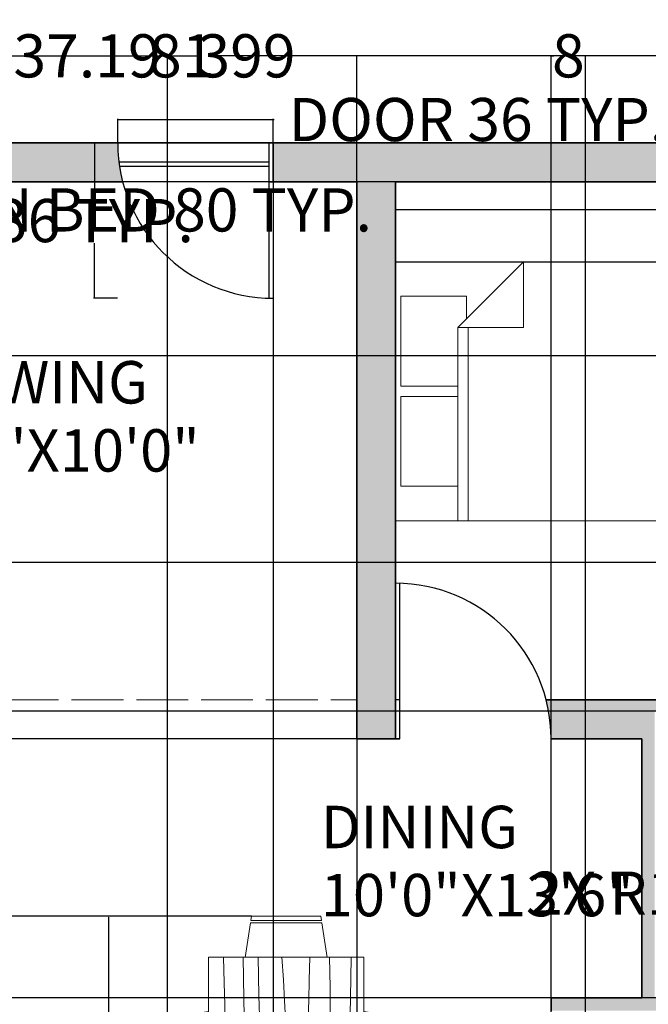
# Model space of a CAD drawing. Units: inches. Extents: x -75 to 484, y -248 to 214.
# Tile 6 of 7: x 162 to 308, y -52 to 176. Entities that reach past the tile are written whole.
import ezdxf

# ---------------------------------------------------------------- set-up
doc = ezdxf.new("R2010")
doc.units = ezdxf.units.IN
doc.header["$MEASUREMENT"] = 0
doc.linetypes.add('ACAD_ISO02W100', pattern=[15, 12, -3])
for name, color, linetype, lineweight in [('A-ANNO-DIMS', 2, 'Continuous', 18), ('A-AREA-IDEN', 7, 'Continuous', 18), ('A-DOOR', 3, 'Continuous', 25), ('A-FURN', 8, 'Continuous', 18), ('A-WALL', 7, 'Continuous', 35), ('A-WALL-OVHD', 7, 'ACAD_ISO02W100', 18)]:
    doc.layers.add(name, color=color, linetype=linetype, lineweight=lineweight)
doc.layers.add('A-WALL-PATT', color=252, linetype='Continuous', lineweight=9, true_color=0x939598)
doc.styles.get("Standard").update_dxf_attribs({"font": 'arial.ttf'})
doc.dimstyles.get("Standard").update_dxf_attribs({"dimtxt": 10, "dimasz": 0.18, "dimexe": 0.18, "dimexo": 0.0625, "dimgap": 0.09, "dimtad": 0, "dimtih": 1, "dimtoh": 1, "dimdec": 0, "dimzin": 0, "dimdsep": 46, "dimlunit": 3, "dimtxsty": 'Standard', "dimcen": 0.09, "dimadec": 0, "dimazin": 0, "dimtfac": 1, "dimtdec": 0, "dimtofl": 0, "dimtmove": 0, "dimatfit": 3, "dimfxl": 1, "dimtolj": 1, "dimtzin": 0, "dimarcsym": 0})

# ---------------------------------------------------------------- blocks, each defined once
blk = doc.blocks.new('Bed - Queen')
for p, q in [((0, -80.00003), (0, 0)), ((0, 0), (59.99999, 0)), ((59.99999, 0), (59.99999, -80.00003)), ((7.99999, -1.2), (28.79998, -1.2)), ((7.99999, -14.4), (7.99999, -1.2)), ((28.79998, -1.2), (28.79998, -14.4)), ((31.19999, -1.2), (51.99999, -1.2)), ((31.19999, -14.4), (31.19999, -1.2)), ((51.99999, -1.2), (51.99999, -16.4)), ((0, -14.4), (44.8, -14.4)), ((59.99999, -29.6), (44.8, -14.4)), ((44.8, -14.4), (44.8, -29.6)), ((44.8, -16.8), (0, -16.8)), ((51.99999, -16.4), (46.79936, -16.4)), ((44.8, -29.6), (59.99999, -29.6)), ((59.99999, -80.00003), (0, -80.00003))]:
    blk.add_line(p, q)
blk = doc.blocks.new('Dining Set - 36 x 72 in.')
for p, q in [((-22, 27.5), (-22.1562, 26.50042)), ((-22, 27.5), (-6, 27.5)), ((-5.8437, 26.49966), (-6, 27.5)), ((6, 27.5), (5.8438, 26.50042)), ((6, 27.5), (22, 27.5)), ((22.1563, 26.49966), (22, 27.5)), ((-22.2343, 26.00059), (-23.4847, 17.99762)), ((-22.2304, 26), (-5.7608, 26)), ((-5.8416, 26.5), (-22.1534, 26.5)), ((-4.5152, 17.99762), (-5.7655, 25.99926)), ((5.7657, 26.00059), (4.5153, 17.99762)), ((5.7696, 26), (22.2392, 26)), ((22.1584, 26.5), (5.8466, 26.5)), ((23.4848, 17.99762), (22.2345, 25.99926)), ((36, 18), (-36, 18)), ((-36, 18), (-36, -18)), ((36, -18), (36, 18)), ((-44.0006, 8.23428), (-35.9976, 9.48474)), ((44.0006, 8.23428), (35.9976, 9.48474)), ((-45.5, 8), (-44.5004, 8.15617)), ((-45.5, 8), (-45.5, -8)), ((-44.5, -8.15843), (-44.5, 8.15338)), ((-44, 8.23041), (-44, -8.23915)), ((44, 8.23041), (44, -8.23915)), ((44.5, -8.15843), (44.5, 8.15338)), ((45.5, 8), (44.5005, 8.15617)), ((45.5, 8), (45.5, -8)), ((-44.4997, -8.15631), (-45.5, -8)), ((-35.9976, -9.48476), (-43.9993, -8.2345)), ((35.9976, -9.48476), (43.9993, -8.2345)), ((44.4997, -8.15631), (45.5, -8)), ((-36, -18), (36, -18)), ((-22.2343, -26.0006), (-23.4847, -17.99762)), ((-4.5152, -17.99762), (-5.7655, -25.99928)), ((5.7657, -26.0006), (4.5153, -17.99762)), ((23.4848, -17.99762), (22.2345, -25.99928)), ((-22.2304, -26), (-5.7608, -26)), ((-22, -27.5), (-22.1562, -26.50044)), ((-5.8416, -26.5), (-22.1534, -26.5)), ((-5.8437, -26.49967), (-6, -27.5)), ((5.7696, -26), (22.2392, -26)), ((6, -27.5), (5.8438, -26.50044)), ((22.1584, -26.5), (5.8466, -26.5)), ((22.1563, -26.49967), (22, -27.5)), ((-22, -27.5), (-6, -27.5)), ((6, -27.5), (22, -27.5))]:
    blk.add_line(p, q)
for points in [[(-36, 15), (-31.1772, 14.97754), (-26.8079, 14.91406), (-22.8538, 14.81543), (-19.276, 14.6875), (-16.0362, 14.53613), (-13.0957, 14.36718), (-10.4159, 14.18652), (-7.9583, 14), (-5.6904, 13.81315), (-3.6035, 13.63021), (-1.6954, 13.45508), (0.0365, 13.29166), (1.5945, 13.14388), (2.9811, 13.01562), (4.1988, 12.9108), (5.25, 12.83333), (6.1393, 12.78613), (6.8802, 12.76823), (7.4883, 12.77767), (7.9792, 12.8125), (8.3685, 12.87077), (8.6719, 12.95052), (8.9049, 13.0498), (9.0833, 13.16666), (9.2205, 13.29899), (9.3216, 13.44401), (9.3895, 13.59879), (9.4271, 13.76041), (9.4373, 13.92594), (9.4232, 14.09245), (9.3875, 14.257), (9.3333, 14.41666), (9.2638, 14.56917), (9.1836, 14.71484), (9.0975, 14.85465), (9.0104, 14.98958), (8.9272, 15.1206), (8.8529, 15.2487), (8.7922, 15.37483), (8.75, 15.5), (8.7305, 15.62467), (8.7344, 15.74739), (8.7617, 15.86621), (8.8125, 15.97916), (8.8867, 16.08431), (8.9844, 16.17968), (9.1055, 16.26334), (9.25, 16.33333), (9.4189, 16.38802), (9.6172, 16.42708), (9.8506, 16.45052), (10.125, 16.45833), (10.4463, 16.45052), (10.8203, 16.42708), (11.2529, 16.38802), (11.75, 16.33333), (12.3184, 16.26318), (12.9694, 16.17838), (13.7151, 16.07991), (14.5677, 15.96875), (15.5395, 15.84586), (16.6426, 15.71224), (17.8893, 15.56884), (19.2917, 15.41666), (20.859, 15.25667), (22.5879, 15.08984), (24.4721, 14.91715), (26.5052, 14.73958), (28.6809, 14.5581), (30.9929, 14.3737), (33.4347, 14.18733), (36, 14)], [(-36, 10), (-28.9766, 10.14274), (-23.1725, 10.20442), (-18.4241, 10.19775), (-14.5677, 10.13541), (-11.4399, 10.03011), (-8.877, 9.89453), (-6.7154, 9.74137), (-4.7917, 9.58333), (-2.9698, 9.43082), (-1.2246, 9.28515), (0.4415, 9.14534), (2.026, 9.01041), (3.5266, 8.87939), (4.9408, 8.7513), (6.266, 8.62516), (7.5, 8.5), (8.6411, 8.37549), (9.6914, 8.2539), (10.6538, 8.13818), (11.5312, 8.03125), (12.3267, 7.93603), (13.043, 7.85547), (13.6831, 7.79248), (14.25, 7.75), (14.7471, 7.7303), (15.1797, 7.73307), (15.5537, 7.75732), (15.875, 7.80208), (16.1494, 7.86637), (16.3828, 7.94922), (16.5811, 8.04964), (16.75, 8.16666), (16.8944, 8.29915), (17.0143, 8.44531), (17.1089, 8.60319), (17.1771, 8.77083), (17.218, 8.94629), (17.2305, 9.1276), (17.2137, 9.31282), (17.1667, 9.5), (17.0895, 9.6875), (16.987, 9.875), (16.8649, 10.0625), (16.7292, 10.25), (16.5856, 10.4375), (16.4401, 10.625), (16.2985, 10.8125), (16.1667, 11), (16.05, 11.18733), (15.9518, 11.3737), (15.8752, 11.5581), (15.8229, 11.73958), (15.798, 11.91715), (15.8034, 12.08984), (15.842, 12.25667), (15.9167, 12.41666), (16.0295, 12.56836), (16.1784, 12.70833), (16.3605, 12.83268), (16.5729, 12.9375), (16.8127, 13.01888), (17.0768, 13.07291), (17.3625, 13.0957), (17.6667, 13.08333), (17.9894, 13.03312), (18.3418, 12.94726), (18.7382, 12.82918), (19.1927, 12.68229), (19.7195, 12.51001), (20.3327, 12.31575), (21.0465, 12.10294), (21.875, 11.875), (22.8357, 11.63354), (23.959, 11.37304), (25.2786, 11.08618), (26.8282, 10.76562), (28.6414, 10.40405), (30.752, 9.99414), (33.1936, 9.52856), (36, 9)], [(-36, 5.5), (-30.7157, 5.3348), (-26.069, 5.20963), (-21.9946, 5.11767), (-18.4271, 5.05208), (-15.3009, 5.00602), (-12.5508, 4.97265), (-10.1112, 4.94515), (-7.9167, 4.91666), (-5.909, 4.88167), (-4.0586, 4.83984), (-2.3429, 4.79215), (-0.7396, 4.73958), (0.7739, 4.6831), (2.22, 4.6237), (3.6213, 4.56233), (5, 4.5), (6.373, 4.43782), (7.7344, 4.3776), (9.0723, 4.32129), (10.375, 4.27083), (11.6309, 4.22819), (12.8281, 4.19531), (13.9551, 4.17415), (15, 4.16666), (15.954, 4.17448), (16.819, 4.19791), (17.6001, 4.23698), (18.3021, 4.29166), (18.9299, 4.36198), (19.4883, 4.44791), (19.9823, 4.54948), (20.4167, 4.66666), (20.7969, 4.79899), (21.1302, 4.94401), (21.4245, 5.09879), (21.6875, 5.26041), (21.9271, 5.42594), (22.1511, 5.59245), (22.3672, 5.757), (22.5834, 5.91666), (22.8065, 6.06868), (23.0404, 6.21093), (23.2879, 6.34147), (23.5521, 6.45833), (23.8358, 6.55957), (24.142, 6.64323), (24.4735, 6.70735), (24.8334, 6.75), (25.2235, 6.76969), (25.642, 6.76692), (26.0858, 6.74267), (26.5521, 6.69791), (27.0379, 6.63362), (27.5404, 6.55078), (28.0565, 6.45036), (28.5834, 6.33333), (29.1242, 6.19987), (29.7071, 6.04687), (30.3661, 5.87044), (31.1354, 5.66666), (32.0493, 5.43164), (33.142, 5.16146), (34.4475, 4.85221), (36, 4.5)], [(-36, -1), (-30.7915, -0.6591), (-26.0195, -0.38216), (-21.6519, -0.16284), (-17.6563, 0.00521), (-14.0005, 0.12833), (-10.6523, 0.21289), (-7.5796, 0.26522), (-4.75, 0.29166), (-2.134, 0.29793), (0.2878, 0.28711), (2.5317, 0.26163), (4.6146, 0.22396), (6.5529, 0.17651), (8.3633, 0.12174), (10.0623, 0.06209), (11.6667, 0), (13.1899, -0.06201), (14.6341, -0.1211), (15.9982, -0.17432), (17.2813, -0.21875), (18.4823, -0.25147), (19.6003, -0.26953), (20.6343, -0.27002), (21.5834, -0.25), (22.4481, -0.20768), (23.2357, -0.14584), (23.9549, -0.06836), (24.6146, 0.02083), (25.2235, 0.11784), (25.7904, 0.21875), (26.3241, 0.31966), (26.8334, 0.41666), (27.3265, 0.50618), (27.8099, 0.58593), (28.2894, 0.65397), (28.7709, 0.70833), (29.2601, 0.74707), (29.763, 0.76823), (30.2855, 0.76985), (30.8334, 0.75), (31.4088, 0.70784), (31.9994, 0.64713), (32.589, 0.57275), (33.1615, 0.48958), (33.7008, 0.4025), (34.1908, 0.3164), (34.6153, 0.23616), (34.9584, 0.16666), (35.2099, 0.11165), (35.3848, 0.07031), (35.504, 0.04069), (35.5886, 0.02083), (35.6594, 0.00879), (35.7377, 0.0026), (35.8442, 0.00032), (36, 0)], [(-36, -6.5), (-27.1843, -6.31267), (-20.084, -6.1263), (-14.469, -5.9419), (-10.1094, -5.76042), (-6.7752, -5.58285), (-4.2363, -5.41016), (-2.2629, -5.24333), (-0.625, -5.08334), (0.8708, -4.93099), (2.2715, -4.78646), (3.5872, -4.64974), (4.8281, -4.52084), (6.0046, -4.39974), (7.127, -4.28646), (8.2053, -4.18099), (9.25, -4.08334), (10.2705, -3.99382), (11.2734, -3.91407), (12.2647, -3.84603), (13.25, -3.79167), (14.2354, -3.75293), (15.2266, -3.73177), (16.2295, -3.73015), (17.25, -3.75), (18.2912, -3.79248), (19.3451, -3.85547), (20.4009, -3.93604), (21.4479, -4.03125), (22.4754, -4.13819), (23.4727, -4.25391), (24.4289, -4.37549), (25.3334, -4.5), (26.1785, -4.62492), (26.9694, -4.74935), (27.7145, -4.87281), (28.4219, -4.99479), (29.1, -5.11483), (29.7572, -5.23242), (30.4016, -5.34709), (31.0417, -5.45834), (31.6837, -5.56437), (32.3262, -5.65821), (32.9658, -5.73153), (33.599, -5.77604), (34.2224, -5.78345), (34.8327, -5.74545), (35.4264, -5.65373), (36, -5.5)], [(-36, -10), (-26.4022, -9.81299), (-18.4675, -9.62891), (-11.9839, -9.45069), (-6.7396, -9.28125), (-2.5226, -9.12354), (0.8789, -8.98047), (3.6769, -8.85498), (6.0833, -8.75), (8.2767, -8.66765), (10.3021, -8.60677), (12.1712, -8.56543), (13.8958, -8.54167), (15.4876, -8.53353), (16.9583, -8.53907), (18.3197, -8.55632), (19.5834, -8.58334), (20.7616, -8.61841), (21.8685, -8.66081), (22.9188, -8.71004), (23.9271, -8.76563), (24.9081, -8.82707), (25.8763, -8.89388), (26.8465, -8.96558), (27.8334, -9.04167), (28.8474, -9.12118), (29.8828, -9.20117), (30.93, -9.27824), (31.9792, -9.34896), (33.0205, -9.40991), (34.0443, -9.45768), (35.0407, -9.48885), (36, -9.5)], [(-36, -14.5), (-30.0881, -14.33513), (-25.0332, -14.21224), (-20.7312, -14.12647), (-17.0781, -14.07292), (-13.97, -14.04671), (-11.3027, -14.04297), (-8.9724, -14.05681), (-6.875, -14.08334), (-4.9224, -14.11833), (-3.0905, -14.16016), (-1.3709, -14.20785), (0.2448, -14.26042), (1.7647, -14.3169), (3.1973, -14.3763), (4.5507, -14.43767), (5.8333, -14.5), (7.0554, -14.5621), (8.235, -14.62175), (9.3922, -14.67652), (10.5469, -14.72396), (11.7192, -14.76164), (12.929, -14.78711), (14.1965, -14.79794), (15.5417, -14.79167), (16.9933, -14.76424), (18.6152, -14.70508), (20.4804, -14.60197), (22.6615, -14.44271), (25.2312, -14.21509), (28.2624, -13.9069), (31.8277, -13.50594), (36, -13)]]:
    blk.add_lwpolyline(points)
blk = doc.blocks.new('DOOR-SINGLE-36')
for p, q in [((35, 36), (35, 0)), ((36, 36), (36, 0))]:
    blk.add_line(p, q)
blk.add_arc((36, 36), 36, 180, 270)
blk = doc.blocks.new('*D13')
at = {"layer": 'A-ANNO-DIMS', "color": 0, "lineweight": -2, "transparency": 16777216}
for p, q in [((184.9, 147.72), (184.9, 153.24)), ((185.08, 153.06), (220.72, 153.06)), ((220.9, 147.72), (220.9, 153.24)), ((220.9, 153.06), (221.08, 153.06))]:
    blk.add_line(p, q, dxfattribs=at)
at = {"layer": 'A-ANNO-DIMS', "color": 0, "transparency": 16777216}
for points in [[(185.08, 153.09), (185.08, 153.03), (184.9, 153.06)], [(220.72, 153.09), (220.72, 153.03), (220.9, 153.06)]]:
    blk.add_solid(points, dxfattribs=at)
at = {"layer": 'Defpoints', "color": 0, "transparency": 16777216}
for p in [(220.9, 153.06), (184.9, 147.66), (220.9, 147.66)]:
    blk.add_point(p, dxfattribs=at)
at = {"layer": 'A-ANNO-DIMS', "color": 0, "transparency": 16777216, "insert": (268.16, 153.06), "char_height": 10, "attachment_point": 5}
blk.add_mtext('\\A1;DOOR 36 TYP.', dxfattribs=at)
blk = doc.blocks.new('*D14')
at = {"layer": 'A-ANNO-DIMS', "color": 0, "lineweight": -2, "transparency": 16777216}
for p, q in [((184.84, 147.66), (179.32, 147.66)), ((179.5, 147.48), (179.5, 134.86)), ((179.5, 111.84), (179.5, 124.46)), ((184.84, 111.66), (179.32, 111.66))]:
    blk.add_line(p, q, dxfattribs=at)
at = {"layer": 'A-ANNO-DIMS', "color": 0, "transparency": 16777216}
for points in [[(179.47, 147.48), (179.53, 147.48), (179.5, 147.66)], [(179.47, 111.84), (179.53, 111.84), (179.5, 111.66)]]:
    blk.add_solid(points, dxfattribs=at)
at = {"layer": 'Defpoints', "color": 0, "transparency": 16777216}
for p in [(179.5, 147.66), (184.9, 147.66), (184.9, 111.66)]:
    blk.add_point(p, dxfattribs=at)
at = {"layer": 'A-ANNO-DIMS', "color": 0, "transparency": 16777216, "insert": (179.5, 129.66), "char_height": 10, "attachment_point": 5}
blk.add_mtext('\\A1;36 TYP.', dxfattribs=at)
blk = doc.blocks.new('*D19')
at = {"layer": 'A-ANNO-DIMS', "color": 0, "lineweight": -2, "transparency": 16777216}
for p, q in [((249.21, 120.19), (249.21, 132.31)), ((329.21, 120.19), (329.21, 132.31)), ((249.21, 132.13), (249.03, 132.13)), ((329.03, 132.13), (249.39, 132.13))]:
    blk.add_line(p, q, dxfattribs=at)
at = {"layer": 'A-ANNO-DIMS', "color": 0, "transparency": 16777216}
for points in [[(249.39, 132.16), (249.39, 132.1), (249.21, 132.13)], [(329.03, 132.16), (329.03, 132.1), (329.21, 132.13)]]:
    blk.add_solid(points, dxfattribs=at)
at = {"layer": 'Defpoints', "color": 0, "transparency": 16777216}
for p in [(249.21, 132.13), (249.21, 120.13), (329.21, 120.13)]:
    blk.add_point(p, dxfattribs=at)
at = {"layer": 'A-ANNO-DIMS', "color": 0, "transparency": 16777216, "insert": (181.53, 132.13), "char_height": 10, "attachment_point": 5}
blk.add_mtext('\\A1;QUEEN BED 80 TYP.', dxfattribs=at)
blk = doc.blocks.new('*D27')
at = {"layer": 'A-ANNO-DIMS', "color": 0, "lineweight": -2, "transparency": 16777216}
for p, q in [((196.34, -31.46), (182.57, -31.46)), ((182.75, -31.64), (182.75, -71.7)), ((182.75, -122.28), (182.75, -82.22)), ((196.34, -122.46), (182.57, -122.46))]:
    blk.add_line(p, q, dxfattribs=at)
at = {"layer": 'A-ANNO-DIMS', "color": 0, "transparency": 16777216}
for points in [[(182.72, -31.64), (182.78, -31.64), (182.75, -31.46)], [(182.72, -122.28), (182.78, -122.28), (182.75, -122.46)]]:
    blk.add_solid(points, dxfattribs=at)
at = {"layer": 'Defpoints', "color": 0, "transparency": 16777216}
for p in [(196.4, -31.46), (182.75, -122.46), (196.4, -122.46)]:
    blk.add_point(p, dxfattribs=at)
at = {"layer": 'A-ANNO-DIMS', "color": 0, "transparency": 16777216, "insert": (182.75, -76.96), "char_height": 10, "attachment_point": 5}
blk.add_mtext('\\A1;DINING SET 91', dxfattribs=at)
blk = doc.blocks.new('*D41')
at = {"layer": 'A-ANNO-DIMS', "color": 0, "lineweight": -2, "transparency": 16777216}
for p, q in [((15.21, 147.72), (15.21, 167.99)), ((15.39, 167.81), (203.57, 167.81)), ((414.03, 167.81), (225.85, 167.81)), ((414.21, 147.72), (414.21, 167.99))]:
    blk.add_line(p, q, dxfattribs=at)
at = {"layer": 'A-ANNO-DIMS', "color": 0, "transparency": 16777216}
for points in [[(15.39, 167.84), (15.39, 167.78), (15.21, 167.81)], [(414.03, 167.84), (414.03, 167.78), (414.21, 167.81)]]:
    blk.add_solid(points, dxfattribs=at)
at = {"layer": 'Defpoints', "color": 0, "transparency": 16777216}
for p in [(414.21, 167.81), (15.21, 147.66), (414.21, 147.66)]:
    blk.add_point(p, dxfattribs=at)
at = {"layer": 'A-ANNO-DIMS', "color": 0, "transparency": 16777216, "insert": (214.71, 167.81), "char_height": 10, "attachment_point": 5}
blk.add_mtext('\\A1;399', dxfattribs=at)
blk = doc.blocks.new('*D43')
at = {"layer": 'A-ANNO-DIMS', "color": 0, "lineweight": -2, "transparency": 16777216}
for p, q in [((220.9, 147.59), (220.9, -241.67)), ((240.21, 138.59), (240.21, -241.67)), ((221.08, -241.49), (240.03, -241.49)), ((240.21, -241.49), (240.39, -241.49))]:
    blk.add_line(p, q, dxfattribs=at)
at = {"layer": 'A-ANNO-DIMS', "color": 0, "transparency": 16777216}
for points in [[(221.08, -241.46), (221.08, -241.52), (220.9, -241.49)], [(240.03, -241.46), (240.03, -241.52), (240.21, -241.49)]]:
    blk.add_solid(points, dxfattribs=at)
at = {"layer": 'Defpoints', "color": 0, "transparency": 16777216}
for p in [(220.9, 147.66), (240.21, 138.66), (240.21, -241.49)]:
    blk.add_point(p, dxfattribs=at)
at = {"layer": 'A-ANNO-DIMS', "color": 0, "transparency": 16777216, "insert": (255.92, -241.49), "char_height": 10, "attachment_point": 5}
blk.add_mtext('\\A1;19.31', dxfattribs=at)
blk = doc.blocks.new('*D50')
at = {"layer": 'A-ANNO-DIMS', "color": 0, "lineweight": -2, "transparency": 16777216}
for p, q in [((405.15, 138.66), (-5.12, 138.66)), ((-4.94, 138.48), (-4.94, 123.68)), ((-4.94, 98.48), (-4.94, 113.28)), ((405.15, 98.3), (-5.12, 98.3))]:
    blk.add_line(p, q, dxfattribs=at)
at = {"layer": 'A-ANNO-DIMS', "color": 0, "transparency": 16777216}
for points in [[(-4.97, 138.48), (-4.91, 138.48), (-4.94, 138.66)], [(-4.97, 98.48), (-4.91, 98.48), (-4.94, 98.3)]]:
    blk.add_solid(points, dxfattribs=at)
at = {"layer": 'Defpoints', "color": 0, "transparency": 16777216}
for p in [(405.21, 138.66), (-4.94, 98.3), (405.21, 98.3)]:
    blk.add_point(p, dxfattribs=at)
at = {"layer": 'A-ANNO-DIMS', "color": 0, "transparency": 16777216, "insert": (-4.94, 118.48), "char_height": 10, "attachment_point": 5}
blk.add_mtext('\\A1;40.35', dxfattribs=at)
blk = doc.blocks.new('*D51')
at = {"layer": 'A-ANNO-DIMS', "color": 0, "lineweight": -2, "transparency": 16777216}
for p, q in [((405.15, 98.3), (-5.12, 98.3)), ((-4.94, 98.12), (-4.94, 79.59)), ((-4.94, 50.66), (-4.94, 69.2)), ((405.15, 50.48), (-5.12, 50.48))]:
    blk.add_line(p, q, dxfattribs=at)
at = {"layer": 'A-ANNO-DIMS', "color": 0, "transparency": 16777216}
for points in [[(-4.97, 98.12), (-4.91, 98.12), (-4.94, 98.3)], [(-4.97, 50.66), (-4.91, 50.66), (-4.94, 50.48)]]:
    blk.add_solid(points, dxfattribs=at)
at = {"layer": 'Defpoints', "color": 0, "transparency": 16777216}
for p in [(405.21, 98.3), (-4.94, 50.48), (405.21, 50.48)]:
    blk.add_point(p, dxfattribs=at)
at = {"layer": 'A-ANNO-DIMS', "color": 0, "transparency": 16777216, "insert": (-4.94, 74.39), "char_height": 10, "attachment_point": 5}
blk.add_mtext('\\A1;47.82', dxfattribs=at)
blk = doc.blocks.new('*D57')
at = {"layer": 'A-ANNO-DIMS', "color": 0, "lineweight": -2, "transparency": 16777216}
for p, q in [((285.21, -212.28), (285.21, 167.99)), ((285.39, 167.81), (285.82, 167.81)), ((293.03, 167.81), (292.59, 167.81)), ((293.21, -212.28), (293.21, 167.99))]:
    blk.add_line(p, q, dxfattribs=at)
at = {"layer": 'A-ANNO-DIMS', "color": 0, "transparency": 16777216}
for points in [[(285.39, 167.84), (285.39, 167.78), (285.21, 167.81)], [(293.03, 167.84), (293.03, 167.78), (293.21, 167.81)]]:
    blk.add_solid(points, dxfattribs=at)
at = {"layer": 'Defpoints', "color": 0, "transparency": 16777216}
for p in [(285.21, 167.81), (285.21, -212.34), (293.21, -212.34)]:
    blk.add_point(p, dxfattribs=at)
at = {"layer": 'A-ANNO-DIMS', "color": 0, "transparency": 16777216, "insert": (289.21, 167.81), "char_height": 10, "attachment_point": 5}
blk.add_mtext('\\A1;8', dxfattribs=at)
blk = doc.blocks.new('*D60')
at = {"layer": 'A-ANNO-DIMS', "color": 0, "lineweight": -2, "transparency": 16777216}
for p, q in [((375.24, 16.05), (-5.12, 16.05)), ((-4.94, 15.87), (-4.94, -11.95)), ((-4.94, -50.16), (-4.94, -22.35)), ((375.24, -50.34), (-5.12, -50.34))]:
    blk.add_line(p, q, dxfattribs=at)
at = {"layer": 'A-ANNO-DIMS', "color": 0, "transparency": 16777216}
for points in [[(-4.97, 15.87), (-4.91, 15.87), (-4.94, 16.05)], [(-4.97, -50.16), (-4.91, -50.16), (-4.94, -50.34)]]:
    blk.add_solid(points, dxfattribs=at)
at = {"layer": 'Defpoints', "color": 0, "transparency": 16777216}
for p in [(375.3, 16.05), (-4.94, -50.34), (375.3, -50.34)]:
    blk.add_point(p, dxfattribs=at)
at = {"layer": 'A-ANNO-DIMS', "color": 0, "transparency": 16777216, "insert": (-4.94, -17.15), "char_height": 10, "attachment_point": 5}
blk.add_mtext('\\A1;66.39', dxfattribs=at)
blk = doc.blocks.new('*D75')
at = {"layer": 'A-ANNO-DIMS', "color": 0, "lineweight": -2, "transparency": 16777216}
for p, q in [((249.27, 138.66), (434.54, 138.66)), ((434.36, 138.48), (434.36, 134.59)), ((434.36, 120.31), (434.36, 124.2)), ((249.27, 120.13), (434.54, 120.13))]:
    blk.add_line(p, q, dxfattribs=at)
at = {"layer": 'A-ANNO-DIMS', "color": 0, "transparency": 16777216}
for points in [[(434.33, 138.48), (434.39, 138.48), (434.36, 138.66)], [(434.33, 120.31), (434.39, 120.31), (434.36, 120.13)]]:
    blk.add_solid(points, dxfattribs=at)
at = {"layer": 'Defpoints', "color": 0, "transparency": 16777216}
for p in [(249.21, 138.66), (249.21, 120.13), (434.36, 120.13)]:
    blk.add_point(p, dxfattribs=at)
at = {"layer": 'A-ANNO-DIMS', "color": 0, "transparency": 16777216, "insert": (434.36, 129.39), "char_height": 10, "attachment_point": 5}
blk.add_mtext('\\A1;18.527', dxfattribs=at)
blk = doc.blocks.new('*D77')
at = {"layer": 'A-ANNO-DIMS', "color": 0, "lineweight": -2, "transparency": 16777216}
for p, q in [((159.21, -53.28), (159.21, 167.99)), ((159.39, 167.81), (160.83, 167.81)), ((196.22, 167.81), (194.77, 167.81)), ((196.4, -54.9), (196.4, 167.99))]:
    blk.add_line(p, q, dxfattribs=at)
at = {"layer": 'A-ANNO-DIMS', "color": 0, "transparency": 16777216}
for points in [[(159.39, 167.84), (159.39, 167.78), (159.21, 167.81)], [(196.22, 167.84), (196.22, 167.78), (196.4, 167.81)]]:
    blk.add_solid(points, dxfattribs=at)
at = {"layer": 'Defpoints', "color": 0, "transparency": 16777216}
for p in [(196.4, 167.81), (159.21, -53.34), (196.4, -54.96)]:
    blk.add_point(p, dxfattribs=at)
at = {"layer": 'A-ANNO-DIMS', "color": 0, "transparency": 16777216, "insert": (177.8, 167.81), "char_height": 10, "attachment_point": 5}
blk.add_mtext('\\A1;37.19', dxfattribs=at)
blk = doc.blocks.new('*D78')
at = {"layer": 'A-ANNO-DIMS', "color": 0, "lineweight": -2, "transparency": 16777216}
for p, q in [((240.15, 9.66), (-5.12, 9.66)), ((-4.94, 9.48), (-4.94, -5.79)), ((-4.94, -31.28), (-4.94, -16.01)), ((215.84, -31.46), (-5.12, -31.46))]:
    blk.add_line(p, q, dxfattribs=at)
at = {"layer": 'A-ANNO-DIMS', "color": 0, "transparency": 16777216}
for points in [[(-4.97, 9.48), (-4.91, 9.48), (-4.94, 9.66)], [(-4.97, -31.28), (-4.91, -31.28), (-4.94, -31.46)]]:
    blk.add_solid(points, dxfattribs=at)
at = {"layer": 'Defpoints', "color": 0, "transparency": 16777216}
for p in [(-4.94, 9.66), (240.21, 9.66), (215.9, -31.46)]:
    blk.add_point(p, dxfattribs=at)
at = {"layer": 'A-ANNO-DIMS', "color": 0, "transparency": 16777216, "insert": (-4.94, -10.9), "char_height": 10, "attachment_point": 5}
blk.add_mtext('\\A1;41.12', dxfattribs=at)
blk = doc.blocks.new('*D81')
at = {"layer": 'A-ANNO-DIMS', "color": 0, "lineweight": -2, "transparency": 16777216}
for p, q in [((159.21, 18.72), (159.21, 167.99)), ((159.39, 167.81), (193.42, 167.81)), ((240.03, 167.81), (206, 167.81)), ((240.21, 18.72), (240.21, 167.99))]:
    blk.add_line(p, q, dxfattribs=at)
at = {"layer": 'A-ANNO-DIMS', "color": 0, "transparency": 16777216}
for points in [[(159.39, 167.84), (159.39, 167.78), (159.21, 167.81)], [(240.03, 167.84), (240.03, 167.78), (240.21, 167.81)]]:
    blk.add_solid(points, dxfattribs=at)
at = {"layer": 'Defpoints', "color": 0, "transparency": 16777216}
for p in [(240.21, 167.81), (159.21, 18.66), (240.21, 18.66)]:
    blk.add_point(p, dxfattribs=at)
at = {"layer": 'A-ANNO-DIMS', "color": 0, "transparency": 16777216, "insert": (199.71, 167.81), "char_height": 10, "attachment_point": 5}
blk.add_mtext('\\A1;81', dxfattribs=at)
blk = doc.blocks.new('*D91')
at = {"layer": 'A-ANNO-DIMS', "color": 0, "lineweight": -2, "transparency": 16777216}
for p, q in [((343.44, -26.11), (350, -26.99)), ((361.32, -28.53), (361.5, -28.53)), ((361.41, -28.62), (361.41, -28.44))]:
    blk.add_line(p, q, dxfattribs=at)
at = {"layer": 'A-ANNO-DIMS', "color": 0, "transparency": 16777216}
blk.add_solid([(350.01, -26.96), (350, -27.02), (350.18, -27.02)], dxfattribs=at)
at = {"layer": 'Defpoints', "color": 0, "transparency": 16777216}
for p in [(350.18, -27.02), (361.41, -28.53)]:
    blk.add_point(p, dxfattribs=at)
at = {"layer": 'A-ANNO-DIMS', "color": 0, "transparency": 16777216, "insert": (310.87, -26.11), "char_height": 10, "attachment_point": 5}
blk.add_mtext('\\A1;2X R11.33', dxfattribs=at)

msp = doc.modelspace()

# ---------------------------------------------------------------- hatches: boundary and pattern name
at = {"layer": 'A-WALL-PATT'}
h = msp.add_hatch(color=256, dxfattribs=at)
h.dxf.hatch_style = 1
h.paths.add_polyline_path([(184.9004, 147.6567), (15.2094, 147.6567), (15.2094, 92.5031), (24.2094, 92.5031), (24.2094, 138.6567), (186.0436, 138.6567, -0.06325422)])
h.paths.add_polyline_path([(414.2094, 147.6567), (249.2094, 147.6567), (220.9004, 147.6567), (220.9004, 138.6567), (240.2094, 138.6567), (240.2094, 18.6567), (240.2094, 9.6567), (249.2094, 9.6567), (249.2094, 45.6567), (249.2094, 138.6567), (405.2094, 138.6567), (405.2094, 98.3029), (414.2094, 98.3029)])
h.paths.add_polyline_path([(159.2094, 18.6567), (24.2094, 18.6567), (24.2094, 44.5861), (15.2094, 44.5861), (15.2094, 9.6567), (15.2094, -3.1791), (24.2094, -3.1791), (24.2094, 9.6567), (132.2094, 9.6567), (132.2094, -50.3433), (83.7394, -50.3433), (83.7394, -53.3433), (132.2094, -53.3433), (159.2094, -53.3433), (159.2094, -50.3433), (135.2094, -50.3433), (135.2094, 9.6567), (159.2094, 9.6567)])
h.paths.add_polyline_path([(53.8898, -50.3433), (24.2094, -50.3433), (24.2094, -27.303), (15.2094, -27.303), (15.2094, -50.3433), (15.2094, -53.3433), (15.2094, -74.0487), (24.2094, -74.0487), (24.2094, -53.3433), (53.7394, -53.3433, -0.02504709)])
h.paths.add_polyline_path([(24.2094, -121.9657), (15.2094, -121.9657), (15.2094, -212.3433), (15.2094, -221.3433), (24.2094, -221.3433), (84.3017, -221.3433), (84.3017, -212.3433), (24.2094, -212.3433)])
h.paths.add_polyline_path([(414.2094, -155.3433), (414.2094, -53.3433), (414.2094, -50.3433), (414.2094, -36.8417), (405.2094, -36.8417), (405.2094, -50.3433), (309.2094, -50.3433), (309.2094, 16.0463), (324.2573, 16.0463), (324.2573, 18.6567), (284.0663, 18.6567, -0.06325422), (285.2094, 9.6567), (306.2094, 9.6567), (306.2094, -50.3433), (285.2094, -50.3433), (285.2094, -53.3433), (309.2094, -53.3433), (405.2094, -53.3433), (405.2094, -212.3433), (293.2094, -212.3433), (293.2094, -158.3433), (293.2094, -145.3433), (300.0339, -145.3433), (300.0339, -142.3433), (285.2094, -142.3433), (159.2094, -142.3433), (159.2094, -89.3433, -0.02086055), (156.2094, -89.218), (156.2094, -212.3433), (131.9001, -212.3433), (131.9001, -221.3433), (156.2094, -221.3433), (165.2094, -221.3433), (285.2094, -221.3433), (288.6713, -221.3433), (293.2094, -221.3433), (405.2094, -221.3433), (414.2094, -221.3433)])
h.paths.add_polyline_path([(165.2094, -212.3433), (165.2094, -151.3433), (285.2094, -151.3433), (285.2094, -212.3433)], flags=16)
h.paths.add_polyline_path([(189.462, -195.5437), (182.159, -190.2838, -0.23606798), (182.5164, -188.0765), (181.7049, -187.4921), (185.5037, -182.2177), (184.648, -181.6013, -0.04492589), (180.0821, -186.3232), (179.2706, -185.7388), (189.206, -171.9443), (190.0174, -172.5287, -0.04492589), (186.9857, -178.3556), (187.8415, -178.9719), (191.6403, -173.6976), (192.4517, -174.282, -0.23606798), (194.432, -173.2435), (201.735, -178.5034, -0.23606798), (201.3776, -180.7107), (202.189, -181.2952, -0.11764706), (192.2537, -195.0897), (191.4423, -194.5053, -0.23606798)], flags=0)
h.paths.add_polyline_path([(253.751, -177.9543), (254.5293, -177.3263, -0.23606798), (254.0517, -175.1419), (261.056, -169.4904, -0.23606798), (263.0902, -170.419), (263.8684, -169.7911), (267.95, -174.8498), (268.7708, -174.1875, -0.04492589), (265.425, -168.5352), (266.2032, -167.9073), (276.8782, -181.1378), (276.0999, -181.7657, -0.04492589), (271.2826, -177.3006), (270.4618, -177.9629), (274.5434, -183.0216), (273.7651, -183.6495, -0.23606798), (274.2427, -185.834), (267.2383, -191.4854, -0.23606798), (265.2042, -190.5568), (264.4259, -191.1848, -0.11764706)], flags=0)
h.paths.add_polyline_path([(405.2094, -142.3433), (336.0339, -142.3433, -0.02086055), (335.9087, -145.3433), (405.2094, -145.3433)], flags=17)
h.paths.add_polyline_path([(414.2094, 50.4831), (405.2094, 50.4831), (405.2094, 18.6567), (354.2573, 18.6567, -0.02178446), (354.1435, 16.0463), (405.2094, 16.0463), (405.2094, -14.6494), (414.2094, -14.6494), (414.2094, 9.6567)])
h.paths.add_polyline_path([(200.2091, -179.9247), (255.2702, -179.9247), (255.2702, -168.0448), (200.2091, -168.0448)], flags=8)
h.paths.add_polyline_path([(200.2352, -167.6036), (249.7883, -167.6036), (249.7883, -155.8804), (200.2352, -155.8804)], flags=8)

# ---------------------------------------------------------------- linework, layer by layer
at = {"layer": 'A-DOOR'}
for p, q in [((220.9004, 147.6567), (184.9004, 147.6567)), ((220.9004, 147.6567), (220.9004, 147.6567)), ((219.9004, 143.1567), (185.1828, 143.1567)), ((219.9004, 142.1567), (185.3231, 142.1567)), ((250.2094, 18.6567), (249.2094, 18.6567)), ((249.2094, 9.6567), (250.2094, 9.6567)), ((250.2094, 9.6567), (249.2094, 9.6567))]:
    msp.add_line(p, q, dxfattribs=at)
at = {"layer": 'A-WALL'}
for p, q in [((220.9004, 147.6567), (220.9004, 138.6567)), ((249.2094, 147.6567), (414.2094, 147.6567)), ((249.2094, 138.6567), (405.2094, 138.6567)), ((249.2094, 9.6567), (249.2094, 138.6567)), ((240.2094, 18.6567), (240.2094, 9.6567)), ((325.2573, 18.6567), (284.0663, 18.6567)), ((240.2094, 9.6567), (249.2094, 9.6567)), ((306.2094, 9.6567), (285.2094, 9.6567)), ((306.2094, -50.3433), (306.2094, 9.6567)), ((285.2094, -53.3433), (285.2094, -50.3433)), ((285.2094, -50.3433), (306.2094, -50.3433))]:
    msp.add_line(p, q, dxfattribs=at)
for points in [[(249.2094, 147.6567), (15.2094, 147.6567), (15.2094, 9.6567)], [(186.0436, 138.6567), (24.2094, 138.6567), (24.2094, 18.6567), (159.2094, 18.6567)], [(240.2094, 18.6567), (240.2094, 138.6567), (219.9004, 138.6567)], [(249.2094, 18.6567), (249.2094, 138.6567)]]:
    msp.add_lwpolyline(points, dxfattribs=at)
at = {"layer": 'A-WALL-OVHD'}
for p, q in [((159.2094, 18.6567), (240.2094, 18.6567)), ((159.2094, 9.6567), (240.2094, 9.6567))]:
    msp.add_line(p, q, dxfattribs=at)

# ---------------------------------------------------------------- block references
at = {"layer": 'A-DOOR'}
msp.add_blockref('DOOR-SINGLE-36', (184.9004, 111.6567), dxfattribs=at)
at = {"layer": 'A-DOOR', "rotation": 180}
msp.add_blockref('DOOR-SINGLE-36', (285.2094, 45.6567), dxfattribs=at)
at = {"layer": 'A-FURN'}
for name, p, rotation in [('Bed - Queen', (249.2094, 60.1301), 90), ('Dining Set - 36 x 72 in.', (223.8986, -76.9627), 270)]:
    msp.add_blockref(name, p, dxfattribs=dict(at, rotation=rotation))

# ---------------------------------------------------------------- texts
at = {"layer": 'A-AREA-IDEN'}
for s, height, p in [('DRAWING', 9.82058, (131.4281, 87.2987)), ('18\'0"X10\'0"', 9.820584, (131.4281, 71.5228)), ('DINING', 9.82058, (231.8986, -15.6868)), ('10\'0"X13\'6"', 9.820584, (231.8986, -31.4627))]:
    msp.add_text(s, height=height, dxfattribs=at).set_placement(p)

# ---------------------------------------------------------------- dimensions: what is measured, and where the dimension line sits
at = {"layer": 'A-ANNO-DIMS'}
dim = msp.add_linear_dim(base=(220.9004, 153.0567), p1=(184.9004, 147.6567), p2=(220.9004, 147.6567), text='DOOR <> TYP.', dimstyle='Standard', override={"dimdec": 0, "dimlfac": 1, "dimrnd": 0, "dimzin": 0, "dimdsep": 46, "dimlunit": 2}, dxfattribs=at)
dim.commit()
dim.dimension.update_dxf_attribs({"geometry": '*D13', "text_midpoint": (268.1554, 153.0567)})
for base, p1, p2, override, picture, middle in [((414.2094, 167.8067), (15.2094, 147.6567), (414.2094, 147.6567), {"dimdec": 0, "dimlfac": 1, "dimrnd": 0, "dimzin": 0, "dimdsep": 46, "dimlunit": 2}, '*D41', (214.7094, 167.8067)), ((196.3986, 167.8067), (159.2094, -53.3433), (196.3986, -54.9627), {"dimdec": 2, "dimlfac": 1, "dimrnd": 0, "dimzin": 0, "dimdsep": 46, "dimlunit": 2}, '*D77', (177.804, 167.8067)), ((240.2094, 167.8067), (159.2094, 18.6567), (240.2094, 18.6567), {"dimdec": 0, "dimlfac": 1, "dimrnd": 0, "dimzin": 0, "dimdsep": 46, "dimlunit": 2}, '*D81', (199.7094, 167.8067)), ((285.2094, 167.8067), (293.2094, -212.3433), (285.2094, -212.3433), {"dimdec": 0, "dimlfac": 1, "dimrnd": 0, "dimzin": 0, "dimdsep": 46, "dimlunit": 2}, '*D57', (289.2094, 167.8067)), ((240.2094, -241.4933), (220.9004, 147.6567), (240.2094, 138.6567), {"dimdec": 2, "dimlfac": 1, "dimrnd": 0, "dimzin": 0, "dimdsep": 46, "dimlunit": 2}, '*D43', (255.916, -241.4933))]:
    dim = msp.add_linear_dim(base=base, p1=p1, p2=p2, dimstyle='Standard', override=override, dxfattribs=at)
    dim.commit()
    dim.dimension.update_dxf_attribs({"geometry": picture, "text_midpoint": middle})
for base, p1, p2, angle, text, picture, middle in [((249.2094, 132.1301), (329.2094, 120.1301), (249.2094, 120.1301), 180, 'QUEEN BED <> TYP.', '*D19', (181.5281, 132.1301)), ((179.5004, 147.6567), (184.9004, 111.6567), (184.9004, 147.6567), 90, '<> TYP.', '*D14', (179.5004, 129.6567)), ((182.7486, -122.4627), (196.3986, -31.4627), (196.3986, -122.4627), 270, 'DINING SET <>', '*D27', (182.7486, -76.9627))]:
    dim = msp.add_linear_dim(base=base, p1=p1, p2=p2, angle=angle, text=text, dimstyle='Standard', override={"dimdec": 0, "dimlfac": 1, "dimrnd": 0, "dimzin": 0, "dimdsep": 46, "dimlunit": 2}, dxfattribs=at)
    dim.commit()
    dim.dimension.update_dxf_attribs({"geometry": picture, "text_midpoint": middle})
for base, p1, p2, override, picture, middle in [((-4.9406, 98.3029), (405.2094, 138.6567), (405.2094, 98.3029), {"dimdec": 2, "dimlfac": 1, "dimrnd": 0, "dimzin": 0, "dimdsep": 46, "dimlunit": 2}, '*D50', (-4.9406, 118.4798)), ((434.3594, 120.1301), (249.2094, 138.6567), (249.2094, 120.1301), {"dimdec": 3, "dimlfac": 1, "dimrnd": 0, "dimzin": 0, "dimdsep": 46, "dimlunit": 2}, '*D75', (434.3594, 129.3934)), ((-4.9406, 50.4831), (405.2094, 98.3029), (405.2094, 50.4831), {"dimdec": 2, "dimlfac": 1, "dimrnd": 0, "dimzin": 0, "dimdsep": 46, "dimlunit": 2}, '*D51', (-4.9406, 74.393)), ((-4.9406, -50.3433), (375.3026, 16.0463), (375.3026, -50.3433), {"dimdec": 2, "dimlfac": 1, "dimrnd": 0, "dimzin": 0, "dimdsep": 46, "dimlunit": 2}, '*D60', (-4.9406, -17.1485)), ((-4.9406, 9.6567), (215.8986, -31.4627), (240.2094, 9.6567), {"dimdec": 2, "dimlfac": 1, "dimrnd": 0, "dimzin": 0, "dimdsep": 46, "dimlunit": 2}, '*D78', (-4.9406, -10.903))]:
    dim = msp.add_linear_dim(base=base, p1=p1, p2=p2, angle=90, dimstyle='Standard', override=override, dxfattribs=at)
    dim.commit()
    dim.dimension.update_dxf_attribs({"geometry": picture, "text_midpoint": middle})
dim = msp.add_radius_dim(center=(361.4093, -28.5259), mpoint=(350.1812, -27.016), text='2X <>', dimstyle='Standard', override={"dimdec": 2, "dimlfac": 1, "dimrnd": 0, "dimzin": 0, "dimdsep": 46, "dimlunit": 2}, dxfattribs=at)
dim.commit()
dim.dimension.update_dxf_attribs({"geometry": '*D91', "text_midpoint": (343.4443, -26.1101), "dimtype": 164})

doc.saveas('drawing.dxf')
